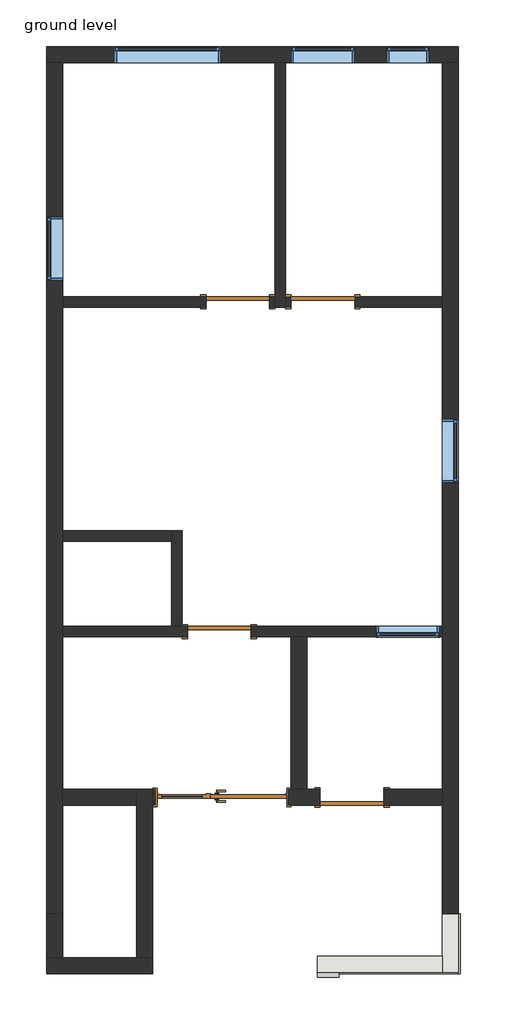
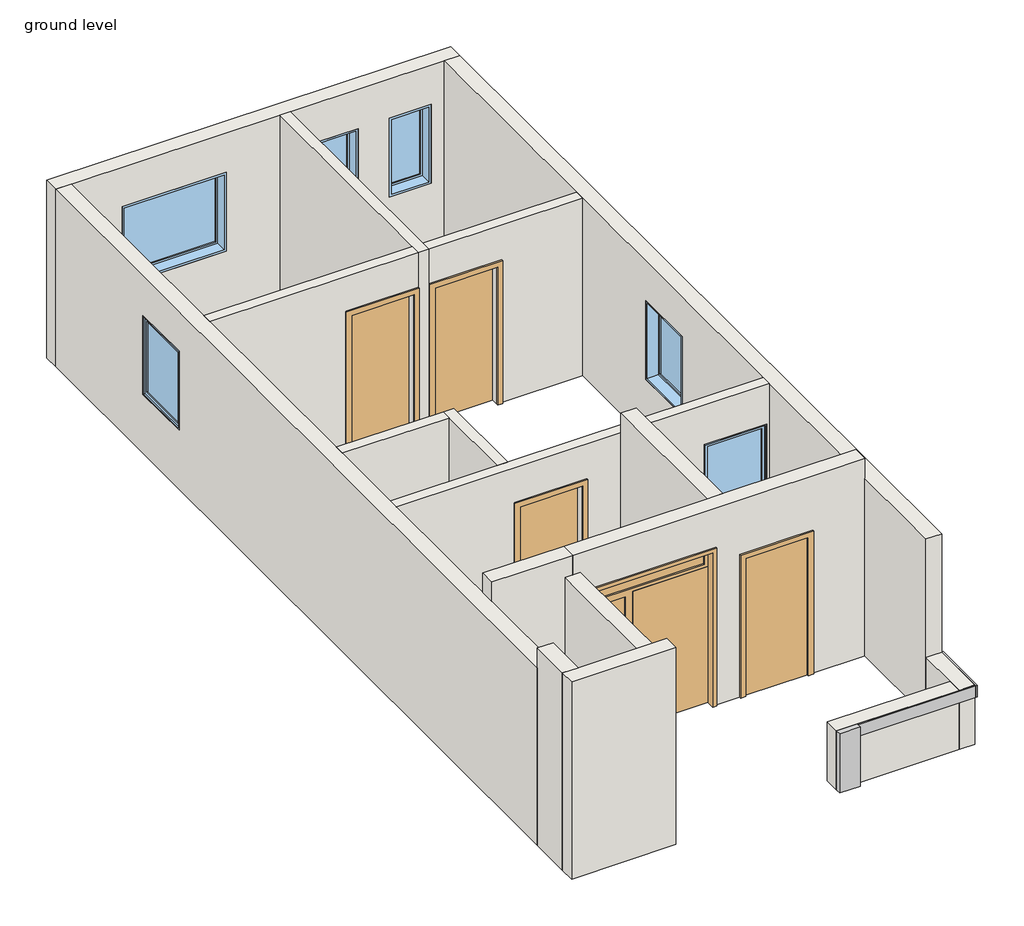
# One storey: 17 walls, 6 windows, 5 doors, 1 column, 1 proxy.
"""IFC4 building model written with IfcOpenShell, lengths in millimetres."""

from ifc_helpers import new_model, si_unit, frame, origin, place, context, project, spatial, polyline, outline, extrude, faceted_brep, transform, mapped, element, save
from components import generic_models_1_generic_models_1_a93b3e87, main_entrance_door_11153_main_entrance_door_11153_7490fc8c, door_686f89d2, door_16372e1c, door_0ca8825f, fixed_2_x3_c82808a1, window_d657a5cb, window_c1f32544, window_145d3b12

model = new_model("IFC4")

# Units and contexts
model_context = context("Model", 3, world=origin())
ifc_project = project(units=[si_unit("LENGTHUNIT", "METRE", prefix="MILLI")], contexts=[model_context])

# Site, building, storey
site = spatial("IfcSite", under=ifc_project)
building = spatial("IfcBuilding", under=site)
storey = spatial("IfcBuildingStorey", under=building, Name="ground level", Elevation=609.6)

# Proxy
placement = place(None, origin())
generic_models_1_generic_models_1_shape = generic_models_1_generic_models_1_a93b3e87(model_context)
element("IfcBuildingElementProxy", 1, Name="Generic Models 1 : Generic Models 1", ObjectType="Generic Models 1 : Generic Models 1", at=placement, inside=storey, context=model_context, shape_type="MappedRepresentation", body=[
    mapped(generic_models_1_generic_models_1_shape, transform((0.0, 0.0, 0.0), x_axis=(1.0, 0.0, 0.0), y_axis=(0.0, 1.0, 0.0), z_axis=(0.0, 0.0, 1.0))),
])

# Column
element("IfcColumn", 2, ObjectType="Rectangular Column : 1'x1'", at=placement, inside=storey, context=model_context, shape_type="SweptSolid", body=[
    extrude(outline(polyline([(-12235.5371373, -3431.061407), (-12540.3371373, -3431.061407), (-12540.3371373, -3354.861407), (-12235.5371373, -3354.861407), (-12235.5371373, -3431.061407)])), frame((0.0, 0.0, 609.6), z_axis=(0.0, 0.0, 1.0), x_axis=(1.0, 0.0, 0.0)), (0.0, 0.0, 1.0), 914.4),
])

# Doors
main_entrance_door_11153_main_entrance_door_11153_shape = main_entrance_door_11153_main_entrance_door_11153_7490fc8c(model_context)
element("IfcDoor", 3, ObjectType="Main_entrance_door_11153 : Main_entrance_door_11153", at=placement, inside=storey, context=model_context, shape_type="MappedRepresentation", body=[
    mapped(main_entrance_door_11153_main_entrance_door_11153_shape, transform((-13911.9371373, -852.961407, 609.6), x_axis=(-1.0, 0.0, 0.0), y_axis=(0.0, -1.0, 0.0), z_axis=(0.0, 0.0, 1.0))),
])
door_shape = door_686f89d2(model_context)
element("IfcDoor", 4, ObjectType="Single-Flush : 36\" x 84\"", at=placement, inside=storey, context=model_context, shape_type="MappedRepresentation", body=[
    mapped(door_shape, transform((-13950.0371373, 1521.938593, 609.6), x_axis=(-1.0, 0.0, 0.0), y_axis=(0.0, -1.0, 0.0), z_axis=(0.0, 0.0, 1.0))),
])
element("IfcDoor", 5, ObjectType="Single-Flush : 36\" x 84\"", at=placement, inside=storey, context=model_context, shape_type="MappedRepresentation", body=[
    mapped(door_shape, transform((-12464.1371373, 6246.338593, 609.6), x_axis=(-1.0, 0.0, 0.0), y_axis=(0.0, -1.0, 0.0), z_axis=(0.0, 0.0, 1.0))),
])
door_2_shape = door_16372e1c(model_context)
element("IfcDoor", 6, ObjectType="Single-Flush : 36\" x 84\"", at=placement, inside=storey, context=model_context, shape_type="MappedRepresentation", body=[
    mapped(door_2_shape, transform((-13683.3371373, 6246.338593, 609.6), x_axis=(1.0, 0.0, 0.0), y_axis=(0.0, 1.0, 0.0), z_axis=(0.0, 0.0, 1.0))),
])
door_3_shape = door_0ca8825f(model_context)
element("IfcDoor", 7, ObjectType="Single-Flush : 36\" x 84\"", at=placement, inside=storey, context=model_context, shape_type="MappedRepresentation", body=[
    mapped(door_3_shape, transform((-12045.0371373, -852.961407, 609.6), x_axis=(-1.0, 0.0, 0.0), y_axis=(0.0, -1.0, 0.0), z_axis=(0.0, 0.0, 1.0))),
])

# Walls
element("IfcWall", 8, ObjectType="wall 6\"", at=placement, inside=storey, context=model_context, shape_type="Brep", body=[
    faceted_brep([(-13149.9371373, 9675.338593, 609.6), (-13149.9371373, 6322.538593, 609.6), (-13149.9371373, 6170.138593, 609.6), (-13149.9371373, 6170.138593, 3352.8), (-13149.9371373, 6322.538593, 3352.8), (-13149.9371373, 9675.338593, 3352.8), (-12997.5371373, 9675.338593, 609.6), (-12997.5371373, 9675.338593, 3352.8), (-12997.5371373, 6322.538593, 3352.8), (-12997.5371373, 6170.138593, 3352.8), (-12997.5371373, 6170.138593, 609.6), (-12997.5371373, 6322.538593, 609.6)], [[[0, 1, 2, 3, 4, 5]], [[6, 7, 8, 9, 10, 11]], [[2, 1, 0, 6, 11, 10]], [[0, 5, 7, 6]], [[3, 2, 10, 9]], [[5, 4, 3, 9, 8, 7]]]),
])
element("IfcWall", 9, ObjectType="wall 6\"", at=placement, inside=storey, context=model_context, shape_type="SweptSolid", body=[
    extrude(outline(polyline([(609.6, -13149.9371373), (3352.8, -13149.9371373), (3352.8, -16197.9371373), (609.6, -16197.9371373), (609.6, -14140.5371373), (2743.2, -14140.5371373), (2743.2, -13226.1371373), (609.6, -13226.1371373), (609.6, -13149.9371373)])), frame((0.0, 6170.138593, 0.0), z_axis=(0.0, 1.0, 0.0), x_axis=(0.0, 0.0, 1.0)), (0.0, 0.0, 1.0), 152.4),
])
element("IfcWall", 10, ObjectType="wall 6\"", at=placement, inside=storey, context=model_context, shape_type="SweptSolid", body=[
    extrude(outline(polyline([(3352.8, -12997.5371373), (609.6, -12997.5371373), (609.6, -12921.3371373), (2743.2, -12921.3371373), (2743.2, -12006.9371373), (609.6, -12006.9371373), (609.6, -10749.6371373), (3352.8, -10749.6371373), (3352.8, -12997.5371373)])), frame((0.0, 6170.138593, 0.0), z_axis=(0.0, 1.0, 0.0), x_axis=(0.0, 0.0, 1.0)), (0.0, 0.0, 1.0), 152.4),
])
element("IfcWall", 11, ObjectType="wall 6\"", at=placement, inside=storey, context=model_context, shape_type="Brep", body=[
    faceted_brep([(-16197.9371373, 1445.738593, 3352.8), (-16197.9371373, 1445.738593, 609.6), (-14407.2371373, 1445.738593, 609.6), (-14407.2371373, 1445.738593, 2743.2), (-13492.8371373, 1445.738593, 2743.2), (-13492.8371373, 1445.738593, 609.6), (-12921.3371373, 1445.738593, 609.6), (-12692.7371373, 1445.738593, 609.6), (-10749.6371373, 1445.738593, 609.6), (-10749.6371373, 1445.738593, 3352.8), (-11702.1371373, 1445.738593, 1524.0), (-11702.1371373, 1445.738593, 2743.2), (-10787.7371373, 1445.738593, 2743.2), (-10787.7371373, 1445.738593, 1524.0), (-16197.9371373, 1598.138593, 609.6), (-16197.9371373, 1598.138593, 3352.8), (-14635.8371373, 1598.138593, 3352.8), (-14483.4371373, 1598.138593, 3352.8), (-10749.6371373, 1598.138593, 3352.8), (-10749.6371373, 1598.138593, 609.6), (-13492.8371373, 1598.138593, 609.6), (-13492.8371373, 1598.138593, 2743.2), (-14407.2371373, 1598.138593, 2743.2), (-14407.2371373, 1598.138593, 609.6), (-14483.4371373, 1598.138593, 609.6), (-14635.8371373, 1598.138593, 609.6), (-11702.1371373, 1598.138593, 2743.2), (-11702.1371373, 1598.138593, 1524.0), (-10787.7371373, 1598.138593, 1524.0), (-10787.7371373, 1598.138593, 2743.2)], [[[0, 1, 2, 3, 4, 5, 6, 7, 8, 9], [10, 11, 12, 13]], [[14, 15, 16, 17, 18, 19, 20, 21, 22, 23, 24, 25], [26, 27, 28, 29]], [[1, 14, 25, 24, 23, 2]], [[19, 8, 7, 6, 5, 20]], [[1, 0, 15, 14]], [[9, 8, 19, 18]], [[0, 9, 18, 17, 16, 15]], [[22, 3, 2, 23]], [[3, 22, 21, 4]], [[4, 21, 20, 5]], [[26, 11, 10, 27]], [[27, 10, 13, 28]], [[28, 13, 12, 29]], [[11, 26, 29, 12]]]),
])
element("IfcWall", 12, ObjectType="wall 6\"", at=placement, inside=storey, context=model_context, shape_type="Brep", body=[
    faceted_brep([(-14483.4371373, 1598.138593, 609.6), (-14483.4371373, 2969.738593, 609.6), (-14483.4371373, 2969.738593, 3352.8), (-14483.4371373, 1598.138593, 3352.8), (-14635.8371373, 1598.138593, 609.6), (-14635.8371373, 1598.138593, 3352.8), (-14635.8371373, 2817.338593, 3352.8), (-14635.8371373, 2969.738593, 3352.8), (-14635.8371373, 2969.738593, 609.6), (-14635.8371373, 2817.338593, 609.6)], [[[0, 1, 2, 3]], [[4, 5, 6, 7, 8, 9]], [[1, 0, 4, 9, 8]], [[0, 3, 5, 4]], [[2, 1, 8, 7]], [[3, 2, 7, 6, 5]]]),
])
element("IfcWall", 13, ObjectType="wall 6\"", at=placement, inside=storey, context=model_context, shape_type="SweptSolid", body=[
    extrude(outline(polyline([(-16197.9371373, 2969.738593), (-14635.8371373, 2969.738593), (-14635.8371373, 2817.338593), (-16197.9371373, 2817.338593), (-16197.9371373, 2969.738593)])), frame((0.0, 0.0, 609.6), z_axis=(0.0, 0.0, 1.0), x_axis=(1.0, 0.0, 0.0)), (0.0, 0.0, 1.0), 2743.2),
])
element("IfcWall", 14, ObjectType="wall 9\"", at=placement, inside=storey, context=model_context, shape_type="Brep", body=[
    faceted_brep([(-16426.5371373, 9675.338593, 609.6), (-16197.9371373, 9675.338593, 609.6), (-13149.9371373, 9675.338593, 609.6), (-12997.5371373, 9675.338593, 609.6), (-10749.6371373, 9675.338593, 609.6), (-10521.0371373, 9675.338593, 609.6), (-10521.0371373, 9675.338593, 3352.8), (-10749.6371373, 9675.338593, 3352.8), (-12997.5371373, 9675.338593, 3352.8), (-13149.9371373, 9675.338593, 3352.8), (-16197.9371373, 9675.338593, 3352.8), (-16426.5371373, 9675.338593, 3352.8), (-13930.9871373, 9675.338593, 2743.2), (-13930.9871373, 9675.338593, 1524.0), (-15454.9871373, 9675.338593, 1524.0), (-15454.9871373, 9675.338593, 2743.2), (-10940.1371373, 9675.338593, 2743.2), (-10940.1371373, 9675.338593, 1524.0), (-11549.7371373, 9675.338593, 1524.0), (-11549.7371373, 9675.338593, 2743.2), (-12006.9371373, 9675.338593, 2743.2), (-12006.9371373, 9675.338593, 1524.0), (-12921.3371373, 9675.338593, 1524.0), (-12921.3371373, 9675.338593, 2743.2), (-10521.0371373, 9903.938593, 609.6), (-16426.5371373, 9903.938593, 609.6), (-16426.5371373, 9903.938593, 3352.8), (-10521.0371373, 9903.938593, 3352.8), (-13930.9871373, 9903.938593, 1524.0), (-13930.9871373, 9903.938593, 2743.2), (-15454.9871373, 9903.938593, 2743.2), (-15454.9871373, 9903.938593, 1524.0), (-10940.1371373, 9903.938593, 1524.0), (-10940.1371373, 9903.938593, 2743.2), (-11549.7371373, 9903.938593, 2743.2), (-11549.7371373, 9903.938593, 1524.0), (-12006.9371373, 9903.938593, 1524.0), (-12006.9371373, 9903.938593, 2743.2), (-12921.3371373, 9903.938593, 2743.2), (-12921.3371373, 9903.938593, 1524.0)], [[[0, 1, 2, 3, 4, 5, 6, 7, 8, 9, 10, 11], [12, 13, 14, 15], [16, 17, 18, 19], [20, 21, 22, 23]], [[24, 25, 26, 27], [28, 29, 30, 31], [32, 33, 34, 35], [36, 37, 38, 39]], [[5, 4, 3, 2, 1, 0, 25, 24]], [[0, 11, 26, 25]], [[6, 5, 24, 27]], [[11, 10, 9, 8, 7, 6, 27, 26]], [[12, 29, 28, 13]], [[13, 28, 31, 14]], [[30, 15, 14, 31]], [[29, 12, 15, 30]], [[16, 33, 32, 17]], [[17, 32, 35, 18]], [[34, 19, 18, 35]], [[33, 16, 19, 34]], [[20, 37, 36, 21]], [[21, 36, 39, 22]], [[22, 39, 38, 23]], [[37, 20, 23, 38]]]),
])
element("IfcWall", 15, ObjectType="wall 9\"", at=placement, inside=storey, context=model_context, shape_type="Brep", body=[
    faceted_brep([(-16426.5371373, 9675.338593, 609.6), (-16426.5371373, -2516.661407, 609.6), (-16426.5371373, -2516.661407, 3352.8), (-16426.5371373, 9675.338593, 3352.8), (-16426.5371373, 7465.538593, 1524.0), (-16426.5371373, 7465.538593, 2743.2), (-16426.5371373, 6551.138593, 2743.2), (-16426.5371373, 6551.138593, 1524.0), (-16197.9371373, -2516.661407, 609.6), (-16197.9371373, -967.261407, 609.6), (-16197.9371373, -738.661407, 609.6), (-16197.9371373, 1445.738593, 609.6), (-16197.9371373, 1598.138593, 609.6), (-16197.9371373, 2817.338593, 609.6), (-16197.9371373, 2969.738593, 609.6), (-16197.9371373, 6170.138593, 609.6), (-16197.9371373, 6322.538593, 609.6), (-16197.9371373, 9675.338593, 609.6), (-16197.9371373, 9675.338593, 3352.8), (-16197.9371373, 6322.538593, 3352.8), (-16197.9371373, 6170.138593, 3352.8), (-16197.9371373, 2969.738593, 3352.8), (-16197.9371373, 2817.338593, 3352.8), (-16197.9371373, 1598.138593, 3352.8), (-16197.9371373, 1445.738593, 3352.8), (-16197.9371373, -2516.661407, 3352.8), (-16197.9371373, 7465.538593, 2743.2), (-16197.9371373, 7465.538593, 1524.0), (-16197.9371373, 6551.138593, 1524.0), (-16197.9371373, 6551.138593, 2743.2)], [[[0, 1, 2, 3], [4, 5, 6, 7]], [[8, 9, 10, 11, 12, 13, 14, 15, 16, 17, 18, 19, 20, 21, 22, 23, 24, 25], [26, 27, 28, 29]], [[1, 0, 17, 16, 15, 14, 13, 12, 11, 10, 9, 8]], [[2, 1, 8, 25]], [[0, 3, 18, 17]], [[3, 2, 25, 24, 23, 22, 21, 20, 19, 18]], [[26, 5, 4, 27]], [[27, 4, 7, 28]], [[28, 7, 6, 29]], [[5, 26, 29, 6]]]),
])
element("IfcWall", 16, ObjectType="wall 9\"", at=placement, inside=storey, context=model_context, shape_type="Brep", body=[
    faceted_brep([(-10749.6371373, 9675.338593, 609.6), (-10749.6371373, 6322.538593, 609.6), (-10749.6371373, 6170.138593, 609.6), (-10749.6371373, 1598.138593, 609.6), (-10749.6371373, 1445.738593, 609.6), (-10749.6371373, -738.661407, 609.6), (-10749.6371373, -967.261407, 609.6), (-10749.6371373, -2516.661407, 609.6), (-10749.6371373, -2516.661407, 1524.0), (-10749.6371373, -2516.661407, 3352.8), (-10749.6371373, 1445.738593, 3352.8), (-10749.6371373, 1598.138593, 3352.8), (-10749.6371373, 6170.138593, 3352.8), (-10749.6371373, 6322.538593, 3352.8), (-10749.6371373, 9675.338593, 3352.8), (-10749.6371373, 3655.538593, 2743.2), (-10749.6371373, 3655.538593, 1524.0), (-10749.6371373, 4569.938593, 1524.0), (-10749.6371373, 4569.938593, 2743.2), (-10521.0371373, -2516.661407, 609.6), (-10521.0371373, 9675.338593, 609.6), (-10521.0371373, 9675.338593, 3352.8), (-10521.0371373, -2516.661407, 3352.8), (-10521.0371373, -2516.661407, 1524.0), (-10521.0371373, 3655.538593, 1524.0), (-10521.0371373, 3655.538593, 2743.2), (-10521.0371373, 4569.938593, 2743.2), (-10521.0371373, 4569.938593, 1524.0)], [[[0, 1, 2, 3, 4, 5, 6, 7, 8, 9, 10, 11, 12, 13, 14], [15, 16, 17, 18]], [[19, 20, 21, 22, 23], [24, 25, 26, 27]], [[7, 6, 5, 4, 3, 2, 1, 0, 20, 19]], [[9, 8, 7, 19, 23, 22]], [[0, 14, 21, 20]], [[14, 13, 12, 11, 10, 9, 22, 21]], [[15, 25, 24, 16]], [[16, 24, 27, 17]], [[17, 27, 26, 18]], [[25, 15, 18, 26]]]),
])
element("IfcWall", 17, ObjectType="wall 9\"", at=placement, inside=storey, context=model_context, shape_type="Brep", body=[
    faceted_brep([(-10749.6371373, -2516.661407, 609.6), (-10749.6371373, -3126.261407, 609.6), (-10749.6371373, -3354.861407, 609.6), (-10749.6371373, -3354.861407, 1524.0), (-10749.6371373, -3126.261407, 1524.0), (-10749.6371373, -2516.661407, 1524.0), (-10521.0371373, -2516.661407, 609.6), (-10521.0371373, -2516.661407, 1524.0), (-10521.0371373, -3354.861407, 1524.0), (-10521.0371373, -3354.861407, 609.6)], [[[0, 1, 2, 3, 4, 5]], [[6, 7, 8, 9]], [[2, 1, 0, 6, 9]], [[5, 4, 3, 8, 7]], [[0, 5, 7, 6]], [[3, 2, 9, 8]]]),
])
element("IfcWall", 18, ObjectType="wall 9\"", at=placement, inside=storey, context=model_context, shape_type="Brep", body=[
    faceted_brep([(-10749.6371373, -3126.261407, 609.6), (-12540.3371373, -3126.261407, 609.6), (-12540.3371373, -3126.261407, 1524.0), (-10749.6371373, -3126.261407, 1524.0), (-10749.6371373, -3354.861407, 609.6), (-10749.6371373, -3354.861407, 1524.0), (-12235.5371373, -3354.861407, 1524.0), (-12540.3371373, -3354.861407, 1524.0), (-12540.3371373, -3354.861407, 609.6), (-12235.5371373, -3354.861407, 609.6)], [[[0, 1, 2, 3]], [[4, 5, 6, 7, 8, 9]], [[1, 0, 4, 9, 8]], [[2, 1, 8, 7]], [[3, 2, 7, 6, 5]], [[0, 3, 5, 4]]]),
])
element("IfcWall", 19, ObjectType="wall 9\"", at=placement, inside=storey, context=model_context, shape_type="Brep", body=[
    faceted_brep([(-16426.5371373, -3380.261407, 609.6), (-14902.5371373, -3380.261407, 609.6), (-14902.5371373, -3380.261407, 3657.6), (-16426.5371373, -3380.261407, 3657.6), (-16426.5371373, -3151.661407, 609.6), (-16426.5371373, -3151.661407, 3657.6), (-16197.9371373, -3151.661407, 3657.6), (-14902.5371373, -3151.661407, 3657.6), (-14902.5371373, -3151.661407, 3352.8), (-14902.5371373, -3151.661407, 609.6), (-15131.1371373, -3151.661407, 609.6), (-16197.9371373, -3151.661407, 609.6)], [[[0, 1, 2, 3]], [[4, 5, 6, 7, 8, 9, 10, 11]], [[1, 0, 4, 11, 10, 9]], [[3, 2, 7, 6, 5]], [[2, 1, 9, 8, 7]], [[0, 3, 5, 4]]]),
])
element("IfcWall", 20, ObjectType="wall 9\"", at=placement, inside=storey, context=model_context, shape_type="Brep", body=[
    faceted_brep([(-14902.5371373, -3151.661407, 609.6), (-14902.5371373, -967.261407, 609.6), (-14902.5371373, -738.661407, 609.6), (-14902.5371373, -738.661407, 3352.8), (-14902.5371373, -967.261407, 3352.8), (-14902.5371373, -3151.661407, 3352.8), (-15131.1371373, -3151.661407, 609.6), (-15131.1371373, -3151.661407, 3352.8), (-15131.1371373, -967.261407, 3352.8), (-15131.1371373, -738.661407, 3352.8), (-15131.1371373, -738.661407, 609.6), (-15131.1371373, -967.261407, 609.6), (-15016.8371373, -738.661407, 3352.8)], [[[0, 1, 2, 3, 4, 5]], [[6, 7, 8, 9, 10, 11]], [[2, 1, 0, 6, 11, 10]], [[5, 4, 3, 12, 9, 8, 7]], [[0, 5, 7, 6]], [[3, 2, 10, 9, 12]]]),
])
element("IfcWall", 21, ObjectType="wall 9\"", at=placement, inside=storey, context=model_context, shape_type="Brep", body=[
    faceted_brep([(-12961.9371373, -967.261407, 609.6), (-12502.2371373, -967.261407, 609.6), (-12502.2371373, -967.261407, 2743.2), (-11587.8371373, -967.261407, 2743.2), (-11587.8371373, -967.261407, 609.6), (-10749.6371373, -967.261407, 609.6), (-10749.6371373, -967.261407, 3657.6), (-15016.8371373, -967.261407, 3657.6), (-15016.8371373, -967.261407, 3352.8), (-14902.5371373, -967.261407, 3352.8), (-14902.5371373, -967.261407, 609.6), (-14861.9371373, -967.261407, 609.6), (-14861.9371373, -967.261407, 3009.6), (-12961.9371373, -967.261407, 3009.6), (-12502.2371373, -738.661407, 2743.2), (-12502.2371373, -738.661407, 609.6), (-12692.7371373, -738.661407, 609.6), (-12921.3371373, -738.661407, 609.6), (-12961.9371373, -738.661407, 609.6), (-12961.9371373, -738.661407, 3009.6), (-14861.9371373, -738.661407, 3009.6), (-14861.9371373, -738.661407, 609.6), (-14902.5371373, -738.661407, 609.6), (-14902.5371373, -738.661407, 3352.8), (-15016.8371373, -738.661407, 3352.8), (-15016.8371373, -738.661407, 3657.6), (-12921.3371373, -738.661407, 3657.6), (-12692.7371373, -738.661407, 3657.6), (-10749.6371373, -738.661407, 3657.6), (-10749.6371373, -738.661407, 609.6), (-11587.8371373, -738.661407, 609.6), (-11587.8371373, -738.661407, 2743.2)], [[[0, 1, 2, 3, 4, 5, 6, 7, 8, 9, 10, 11, 12, 13]], [[14, 15, 16, 17, 18, 19, 20, 21, 22, 23, 24, 25, 26, 27, 28, 29, 30, 31]], [[10, 22, 21, 11]], [[30, 29, 5, 4]], [[18, 17, 16, 15, 1, 0]], [[7, 6, 28, 27, 26, 25]], [[6, 5, 29, 28]], [[20, 12, 11, 21]], [[12, 20, 19, 13]], [[13, 19, 18, 0]], [[7, 25, 24, 8]], [[8, 24, 23, 9]], [[22, 10, 9, 23]], [[2, 1, 15, 14]], [[3, 2, 14, 31]], [[4, 3, 31, 30]]]),
])
element("IfcWall", 22, ObjectType="wall 9\"", at=placement, inside=storey, context=model_context, shape_type="SweptSolid", body=[
    extrude(outline(polyline([(-12692.7371373, 1445.738593), (-12692.7371373, -738.661407), (-12921.3371373, -738.661407), (-12921.3371373, 1445.738593), (-12692.7371373, 1445.738593)])), frame((0.0, 0.0, 609.6), z_axis=(0.0, 0.0, 1.0), x_axis=(1.0, 0.0, 0.0)), (0.0, 0.0, 1.0), 3048.0),
])
element("IfcWall", 23, ObjectType="wall 9\"", at=placement, inside=storey, context=model_context, shape_type="SweptSolid", body=[
    extrude(outline(polyline([(609.6, -15131.1371373), (3352.8, -15131.1371373), (3352.8, -15016.8371373), (3657.6, -15016.8371373), (3657.6, -16197.9371373), (609.6, -16197.9371373), (609.6, -15131.1371373)])), frame((0.0, -967.261407, 0.0), z_axis=(0.0, 1.0, 0.0), x_axis=(0.0, 0.0, 1.0)), (0.0, 0.0, 1.0), 228.6),
])
element("IfcWall", 24, ObjectType="wall 9\"", at=placement, inside=storey, context=model_context, shape_type="Brep", body=[
    faceted_brep([(-16426.5371373, -2516.661407, 609.6), (-16426.5371373, -3151.661407, 609.6), (-16426.5371373, -3151.661407, 3657.6), (-16426.5371373, -2516.661407, 3657.6), (-16426.5371373, -2516.661407, 3352.8), (-16197.9371373, -2516.661407, 609.6), (-16197.9371373, -2516.661407, 3352.8), (-16197.9371373, -2516.661407, 3657.6), (-16197.9371373, -3151.661407, 3657.6), (-16197.9371373, -3151.661407, 609.6)], [[[0, 1, 2, 3, 4]], [[5, 6, 7, 8, 9]], [[1, 0, 5, 9]], [[3, 2, 8, 7]], [[0, 4, 3, 7, 6, 5]], [[2, 1, 9, 8]]]),
])

# Windows
fixed_2_x3_shape = fixed_2_x3_c82808a1(model_context)
element("IfcWindow", 25, ObjectType="Fixed : 24\" x 48\"", at=placement, inside=storey, context=model_context, shape_type="MappedRepresentation", body=[
    mapped(fixed_2_x3_shape, transform((-11206.8371373, 9789.638593, 609.6), x_axis=(1.0, 0.0, 0.0), y_axis=(0.0, 1.0, 0.0), z_axis=(0.0, 0.0, 1.0))),
])
window_shape = window_d657a5cb(model_context)
element("IfcWindow", 26, ObjectType="Fixed : 36\" x 48\"", at=placement, inside=storey, context=model_context, shape_type="MappedRepresentation", body=[
    mapped(window_shape, transform((-11283.0371373, 1521.938593, 609.6), x_axis=(-1.0, 0.0, 0.0), y_axis=(0.0, -1.0, 0.0), z_axis=(0.0, 0.0, 1.0))),
])
window_2_shape = window_c1f32544(model_context)
element("IfcWindow", 27, ObjectType="Fixed : 36\" x 48\"", at=placement, inside=storey, context=model_context, shape_type="MappedRepresentation", body=[
    mapped(window_2_shape, transform((-10635.3371373, 4074.638593, 609.6), x_axis=(0.0, -1.0, 0.0), y_axis=(1.0, 0.0, 0.0), z_axis=(0.0, 0.0, 1.0))),
])
element("IfcWindow", 28, ObjectType="Fixed : 36\" x 48\"", at=placement, inside=storey, context=model_context, shape_type="MappedRepresentation", body=[
    mapped(window_2_shape, transform((-12426.0371373, 9789.638593, 609.6), x_axis=(1.0, 0.0, 0.0), y_axis=(0.0, 1.0, 0.0), z_axis=(0.0, 0.0, 1.0))),
])
element("IfcWindow", 29, ObjectType="Fixed : 36\" x 48\"", at=placement, inside=storey, context=model_context, shape_type="MappedRepresentation", body=[
    mapped(window_2_shape, transform((-16312.2371373, 7046.438593, 609.6), x_axis=(0.0, 1.0, 0.0), y_axis=(-1.0, 0.0, 0.0), z_axis=(0.0, 0.0, 1.0))),
])
window_3_shape = window_145d3b12(model_context)
element("IfcWindow", 30, ObjectType="Fixed : 60\"48", at=placement, inside=storey, context=model_context, shape_type="MappedRepresentation", body=[
    mapped(window_3_shape, transform((-14654.8871373, 9789.638593, 609.6), x_axis=(1.0, 0.0, 0.0), y_axis=(0.0, 1.0, 0.0), z_axis=(0.0, 0.0, 1.0))),
])

save(model, "model.ifc")

# Revit data of these elements
# Type "Rectangular Column : 1'x1'"
#   Assembly Code = "B1010200"
#   Depth = 1' - 0"
#   Offset Base = 0' - 0"
#   Offset Top = 0' - 0"
#   Width = 1' - 0"
#   Material = none
# Type "Main_entrance_door_11153 : Main_entrance_door_11153"
#   Type Mark = "8"
#   Height = 7' - 10.48819"
#   Width = 6' - 2.80315"
#   Door Width = 3' - 7.30709"
#   Function = (empty or 0)
#   Wall Closure = (empty or 0)
# Type "Single-Flush : 36\" x 84\""
#   Type Mark = "1"
#   Construction Type Id = "MDOOR"
#   Assembly Code = "C1020"
#   Analytic Construction = "Metal"
#   Thickness = 0' - 2"
#   Heat Transfer Coefficient (U) = 0.651978 BTU/(h·ft²·°F)
#   Height = 7' - 0"
#   Trim Projection Ext = 0' - 1"
#   Trim Projection Int = 0' - 1"
#   Trim Width = 0' - 3"
#   Width = 3' - 0"
#   Define Thermal Properties by = 1
#   Define Thermal Properties by = 1
#   Door Material = Door - Panel
#   Frame Material = Door - Frame
#   Visual Light Transmittance = 0
#   Solar Heat Gain Coefficient = 0
#   Function = (empty or 0)
#   Wall Closure = (empty or 0)
# Type "wall 6\""
#   Assembly Code = "B2010"
#   Layers, outside or top first: 0' - 6" no material (function 1)
# Type "wall 9\""
#   Assembly Code = "B2010"
#   Layers, outside or top first: 0' - 9" no material (function 1)
# Type "Fixed : 24\" x 48\""
#   Type Mark = "2"
#   Construction Type Id = "GSP4R"
#   Assembly Code = "B2020100"
#   Analytic Construction = "1/8 in Pilkington single glazing"
#   Visual Light Transmittance = 0.9
#   Solar Heat Gain Coefficient = 0.78
#   Heat Transfer Coefficient (U) = 0.6496 BTU/(h·ft²·°F)
#   Height = 4' - 0"
#   Default Sill Height = 3' - 0"
#   Width = 2' - 0"
#   Window Inset = 0' - 0 3/4"
#   Define Thermal Properties by = 1
#   Define Thermal Properties by = 1
#   Glass Pane Material = Glass
#   Sash Material = Sash
#   Wall Closure = (empty or 0)
# Type "Fixed : 36\" x 48\""
#   Type Mark = "1"
#   Construction Type Id = "GSP4R"
#   Assembly Code = "B2020100"
#   Analytic Construction = "1/8 in Pilkington single glazing"
#   Visual Light Transmittance = 0.9
#   Solar Heat Gain Coefficient = 0.78
#   Heat Transfer Coefficient (U) = 0.6496 BTU/(h·ft²·°F)
#   Height = 4' - 0"
#   Default Sill Height = 3' - 0"
#   Width = 3' - 0"
#   Window Inset = 0' - 0 3/4"
#   Define Thermal Properties by = 1
#   Define Thermal Properties by = 1
#   Glass Pane Material = Glass
#   Sash Material = Sash
#   Wall Closure = (empty or 0)
# Type "Fixed : 60\"48"
#   Type Mark = "18"
#   Construction Type Id = "GSP4R"
#   Assembly Code = "B2020100"
#   Analytic Construction = "1/8 in Pilkington single glazing"
#   Visual Light Transmittance = 0.9
#   Solar Heat Gain Coefficient = 0.78
#   Heat Transfer Coefficient (U) = 0.6496 BTU/(h·ft²·°F)
#   Height = 4' - 0"
#   Default Sill Height = 3' - 0"
#   Width = 5' - 0"
#   Window Inset = 0' - 0 3/4"
#   Define Thermal Properties by = 1
#   Glass Pane Material = Glass
#   Sash Material = Sash
#   Wall Closure = (empty or 0)
# Element 1 (IfcBuildingElementProxy, "Generic Models 1 : Generic Models 1")
#   Phase Created = New Construction
#   Materials on its faces: "Gypsum Wall Board"
# Element 2 (IfcColumn, "Rectangular Column : 1'x1'")
#   Phase Created = New Construction
#   Materials on its faces: "Gypsum Wall Board", "Default Wall", "4. WALL PAINT"
# Element 3 (IfcDoor, "Main_entrance_door_11153 : Main_entrance_door_11153")
#   Phase Created = New Construction
#   Materials on its faces: "Glass", "Default"
# Elements 4, 5, 6, 7 (IfcDoor, "Single-Flush : 36\" x 84\"")
#   Phase Created = New Construction
#   Materials on its faces: "Door - Frame", "Door - Panel"
# Elements 8, 9, 10, 11, 12, 13 (IfcWall, "wall 6\"")
#   Top Offset = 0' - 0"
#   Base Offset = 0' - 0"
#   wall height = 9' - 0"
#   Phase Created = New Construction
#   Base Constraint = ground level
#   Top Constraint = 1. slab level
#   Materials on its faces: "Default Wall"
# Elements 14, 15 (IfcWall, "wall 9\"")
#   Top Offset = 0' - 0"
#   Base Offset = 0' - 0"
#   wall height = 9' - 0"
#   Phase Created = New Construction
#   Base Constraint = ground level
#   Top Constraint = 1. slab level
#   Materials on its faces: "Default Wall", "4. WALL PAINT"
# Element 16 (IfcWall, "wall 9\"")
#   Top Offset = 0' - 0"
#   Base Offset = 0' - 0"
#   wall height = 9' - 0"
#   Phase Created = New Construction
#   Base Constraint = ground level
#   Top Constraint = 1. slab level
#   Materials on its faces: "Default Wall", "3. wall paint", "4. WALL PAINT"
# Elements 17, 18 (IfcWall, "wall 9\"")
#   Top Offset = 0' - 0"
#   Base Offset = 0' - 0"
#   wall height = 3' - 0"
#   Phase Created = New Construction
#   Base Constraint = ground level
#   Top Constraint = level 2
#   Materials on its faces: "Default Wall", "4. WALL PAINT", "Gypsum Wall Board"
# Element 19 (IfcWall, "wall 9\"")
#   Top Offset = 7' - 0"
#   Base Offset = 0' - 0"
#   wall height = 10' - 0"
#   Phase Created = New Construction
#   Base Constraint = ground level
#   Top Constraint = level 2
#   Materials on its faces: "Default Wall", "3. wall paint", "4. WALL PAINT"
# Element 20 (IfcWall, "wall 9\"")
#   Top Offset = 6' - 0"
#   Base Offset = 0' - 0"
#   wall height = 9' - 0"
#   Phase Created = New Construction
#   Base Constraint = ground level
#   Top Constraint = level 2
#   Materials on its faces: "Default Wall", "3. wall paint"
# Element 21 (IfcWall, "wall 9\"")
#   Top Offset = 0' - 0"
#   Base Offset = 0' - 0"
#   wall height = 10' - 0"
#   Phase Created = New Construction
#   Base Constraint = ground level
#   Top Constraint = 1. slab level
#   Materials on its faces: "Default Wall", "3. wall paint"
# Elements 22, 23 (IfcWall, "wall 9\"")
#   Top Offset = 0' - 0"
#   Base Offset = 0' - 0"
#   wall height = 10' - 0"
#   Phase Created = New Construction
#   Base Constraint = ground level
#   Top Constraint = 1. slab level
#   Materials on its faces: "Default Wall"
# Element 24 (IfcWall, "wall 9\"")
#   Top Offset = 0' - 0"
#   Base Offset = 0' - 0"
#   wall height = 10' - 0"
#   Phase Created = New Construction
#   Base Constraint = ground level
#   Top Constraint = 1. slab level
#   Materials on its faces: "Default Wall", "4. WALL PAINT"
# Element 25 (IfcWindow, "Fixed : 24\" x 48\"")
#   Mark = "5"
#   Phase Created = New Construction
#   Materials on its faces: "Sash", "Glass"
# Element 26 (IfcWindow, "Fixed : 36\" x 48\"")
#   Mark = "1"
#   Phase Created = New Construction
#   Materials on its faces: "Sash", "Glass"
# Element 27 (IfcWindow, "Fixed : 36\" x 48\"")
#   Mark = "2"
#   Phase Created = New Construction
#   Materials on its faces: "Sash", "Glass"
# Element 28 (IfcWindow, "Fixed : 36\" x 48\"")
#   Mark = "3"
#   Phase Created = New Construction
#   Materials on its faces: "Sash", "Glass"
# Element 29 (IfcWindow, "Fixed : 36\" x 48\"")
#   Mark = "4"
#   Phase Created = New Construction
#   Materials on its faces: "Sash", "Glass"
# Element 30 (IfcWindow, "Fixed : 60\"48")
#   Mark = "6"
#   Phase Created = New Construction
#   Materials on its faces: "Sash", "Glass"
# Materials
#   "Door - Panel": class "Wood", colour RGB 210 159 95, transparency 0, Cost = 0
#   "Door - Frame": colour RGB 118 70 51, transparency 0, Cost = 0
#   "Glass": class "Glass", colour RGB 0 128 192, transparency 0.75, Description = "Soda Lime Glass", Cost = 0
#   "Sash": class "Wood", colour RGB 224 178 126, transparency 0, Cost = 0
#   "Gypsum Wall Board": class "Generic", colour RGB 127 127 127, transparency 0, Description = "Gypsum Wall Board", Cost = 0
#   "Default Wall": colour RGB 128 128 128, transparency 0, Cost = 0
#   "4. WALL PAINT": class "Generic", colour RGB 120 120 120, transparency 0, Cost = 0
#   "Default": colour RGB 127 127 127, transparency 0, Cost = 0
#   "3. wall paint": class "Generic", colour RGB 120 120 120, transparency 0, Cost = 0
